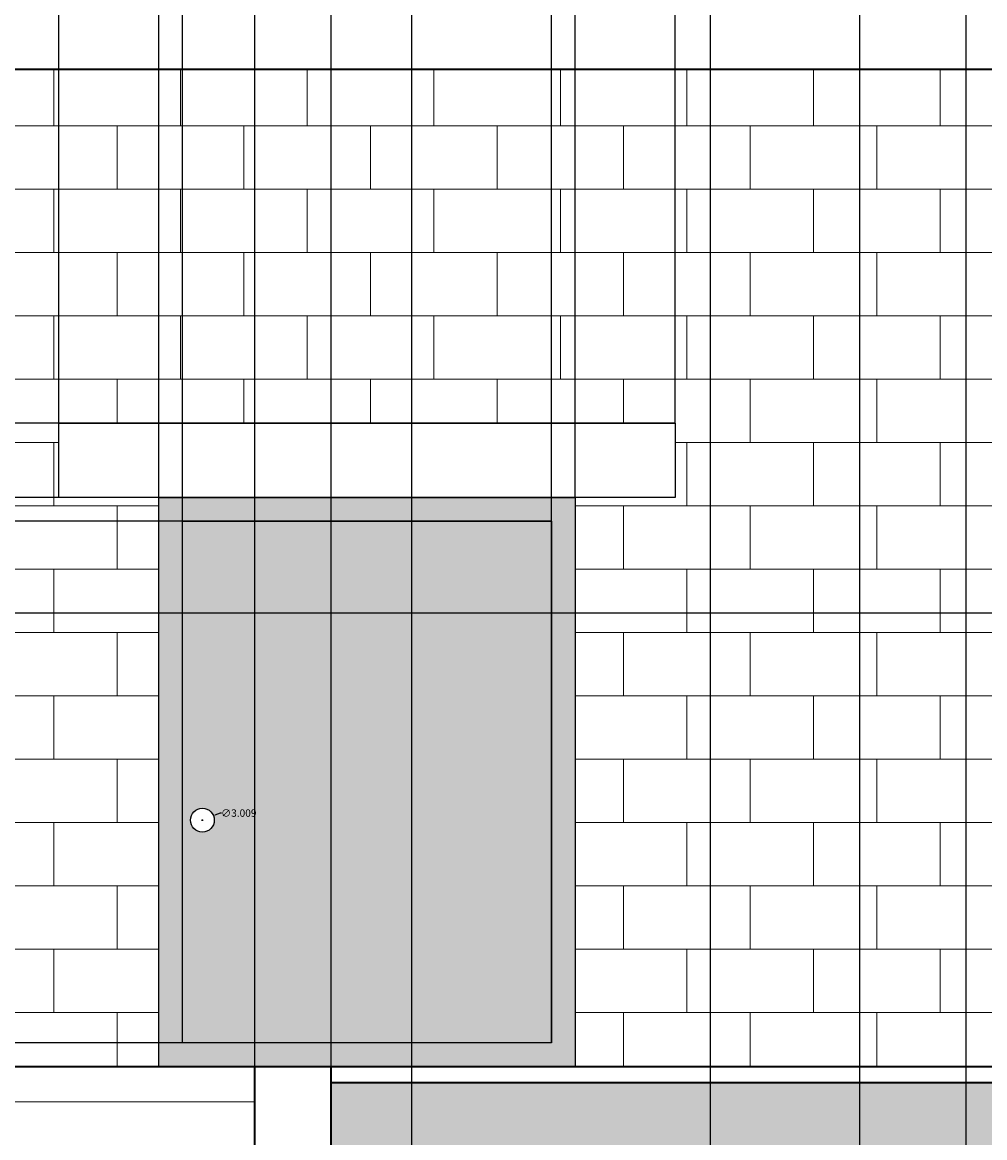
# Model space of a CAD drawing. Units: inches. Extents: x -5 to 714, y 84 to 644.
# Tile 11 of 20: x 220 to 342, y 336 to 477. Entities that reach past the tile are written whole.
import ezdxf

# ---------------------------------------------------------------- set-up
doc = ezdxf.new("R2010")
doc.units = ezdxf.units.IN
doc.header["$MEASUREMENT"] = 0
for name, color, linetype, lineweight in [('A-ANNO-DIMS', 2, 'Continuous', 18), ('A-DOOR', 4, 'Continuous', 25), ('A-ELEV', 7, 'Continuous', 35), ('A-ELEV-PATT', 8, 'Continuous', 13)]:
    doc.layers.add(name, color=color, linetype=linetype, lineweight=lineweight)
doc.styles.get("Standard").update_dxf_attribs({"font": 'arial.ttf'})
doc.dimstyles.get("Standard").update_dxf_attribs({"dimtxt": 0.9375, "dimasz": 0.18, "dimexe": 0.18, "dimexo": 0.0625, "dimgap": 0.09, "dimtad": 0, "dimtih": 1, "dimtoh": 1, "dimdec": 4, "dimzin": 0, "dimdsep": 46, "dimlunit": 4, "dimtxsty": 'Standard', "dimcen": 0.09, "dimadec": 0, "dimazin": 0, "dimtfac": 1, "dimtdec": 4, "dimtofl": 0, "dimtmove": 0, "dimatfit": 3, "dimfxl": 1, "dimtolj": 1, "dimtzin": 0, "dimarcsym": 0})

# ---------------------------------------------------------------- blocks, each defined once
blk = doc.blocks.new('*D27')
at = {"layer": 'A-ANNO-DIMS', "color": 0, "lineweight": -2, "transparency": 16777216}
for p, q in [((429.45, 402.48), (-2.74, 402.48)), ((-2.56, 402.3), (-2.56, 374.41)), ((-2.56, 345.37), (-2.56, 373.27)), ((429.45, 345.19), (-2.74, 345.19))]:
    blk.add_line(p, q, dxfattribs=at)
at = {"layer": 'A-ANNO-DIMS', "color": 0, "transparency": 16777216}
for points in [[(-2.59, 402.3), (-2.53, 402.3), (-2.56, 402.48)], [(-2.59, 345.37), (-2.53, 345.37), (-2.56, 345.19)]]:
    blk.add_solid(points, dxfattribs=at)
at = {"layer": 'Defpoints', "color": 0, "transparency": 16777216}
for p in [(-2.56, 402.48), (429.51, 402.48), (429.51, 345.19)]:
    blk.add_point(p, dxfattribs=at)
at = {"layer": 'A-ANNO-DIMS', "color": 0, "transparency": 16777216, "insert": (-2.56, 373.84), "char_height": 0.938, "attachment_point": 5}
blk.add_mtext('\\A1;57.29', dxfattribs=at)
blk = doc.blocks.new('*D29')
at = {"layer": 'A-ANNO-DIMS', "color": 0, "lineweight": -2, "transparency": 16777216}
for p, q in [((135.73, 471.11), (135.73, 84.31)), ((429.51, 471.11), (429.51, 84.31)), ((135.91, 84.49), (280.94, 84.49)), ((429.33, 84.49), (284.3, 84.49))]:
    blk.add_line(p, q, dxfattribs=at)
at = {"layer": 'A-ANNO-DIMS', "color": 0, "transparency": 16777216}
for points in [[(135.91, 84.52), (135.91, 84.46), (135.73, 84.49)], [(429.33, 84.52), (429.33, 84.46), (429.51, 84.49)]]:
    blk.add_solid(points, dxfattribs=at)
at = {"layer": 'Defpoints', "color": 0, "transparency": 16777216}
for p in [(135.73, 471.17), (429.51, 471.17), (429.51, 84.49)]:
    blk.add_point(p, dxfattribs=at)
at = {"layer": 'A-ANNO-DIMS', "color": 0, "transparency": 16777216, "insert": (282.62, 84.49), "char_height": 0.938, "attachment_point": 5}
blk.add_mtext('\\A1;293.8', dxfattribs=at)
blk = doc.blocks.new('*D31')
at = {"layer": 'A-ANNO-DIMS', "color": 0, "lineweight": -2, "transparency": 16777216}
for p, q in [((135.73, 345.26), (135.73, 643.61)), ((135.91, 643.43), (184.51, 643.43)), ((237.09, 643.43), (188.49, 643.43)), ((237.27, 345.26), (237.27, 643.61))]:
    blk.add_line(p, q, dxfattribs=at)
at = {"layer": 'A-ANNO-DIMS', "color": 0, "transparency": 16777216}
for points in [[(135.91, 643.46), (135.91, 643.4), (135.73, 643.43)], [(237.09, 643.46), (237.09, 643.4), (237.27, 643.43)]]:
    blk.add_solid(points, dxfattribs=at)
at = {"layer": 'Defpoints', "color": 0, "transparency": 16777216}
for p in [(237.27, 643.43), (135.73, 345.19), (237.27, 345.19)]:
    blk.add_point(p, dxfattribs=at)
at = {"layer": 'A-ANNO-DIMS', "color": 0, "transparency": 16777216, "insert": (186.5, 643.43), "char_height": 0.938, "attachment_point": 5}
blk.add_mtext('\\A1;101.54', dxfattribs=at)
blk = doc.blocks.new('*D32')
at = {"layer": 'A-ANNO-DIMS', "color": 0, "lineweight": -2, "transparency": 16777216}
for p, q in [((237.27, 417.15), (237.27, 643.61)), ((237.45, 643.43), (261.91, 643.43)), ((289.7, 643.43), (265.24, 643.43)), ((289.88, 417.15), (289.88, 643.61))]:
    blk.add_line(p, q, dxfattribs=at)
at = {"layer": 'A-ANNO-DIMS', "color": 0, "transparency": 16777216}
for points in [[(237.45, 643.46), (237.45, 643.4), (237.27, 643.43)], [(289.7, 643.46), (289.7, 643.4), (289.88, 643.43)]]:
    blk.add_solid(points, dxfattribs=at)
at = {"layer": 'Defpoints', "color": 0, "transparency": 16777216}
for p in [(289.88, 643.43), (237.27, 417.09), (289.88, 417.09)]:
    blk.add_point(p, dxfattribs=at)
at = {"layer": 'A-ANNO-DIMS', "color": 0, "transparency": 16777216, "insert": (263.57, 643.43), "char_height": 0.938, "attachment_point": 5}
blk.add_mtext('\\A1;52.62', dxfattribs=at)
blk = doc.blocks.new('*D33')
at = {"layer": 'A-ANNO-DIMS', "color": 0, "lineweight": -2, "transparency": 16777216}
for p, q in [((240.27, 348.26), (240.27, 643.61)), ((240.45, 643.43), (261.89, 643.43)), ((286.7, 643.43), (265.26, 643.43)), ((286.88, 348.26), (286.88, 643.61))]:
    blk.add_line(p, q, dxfattribs=at)
at = {"layer": 'A-ANNO-DIMS', "color": 0, "transparency": 16777216}
for points in [[(240.45, 643.46), (240.45, 643.4), (240.27, 643.43)], [(286.7, 643.46), (286.7, 643.4), (286.88, 643.43)]]:
    blk.add_solid(points, dxfattribs=at)
at = {"layer": 'Defpoints', "color": 0, "transparency": 16777216}
for p in [(286.88, 643.43), (240.27, 348.19), (286.88, 348.19)]:
    blk.add_point(p, dxfattribs=at)
at = {"layer": 'A-ANNO-DIMS', "color": 0, "transparency": 16777216, "insert": (263.57, 643.43), "char_height": 0.938, "attachment_point": 5}
blk.add_mtext('\\A1;46.62', dxfattribs=at)
blk = doc.blocks.new('*D34')
at = {"layer": 'A-ANNO-DIMS', "color": 0, "lineweight": -2, "transparency": 16777216}
for p, q in [((286.82, 414.09), (-2.74, 414.09)), ((-2.56, 413.91), (-2.56, 381.71)), ((-2.56, 348.37), (-2.56, 380.57)), ((286.82, 348.19), (-2.74, 348.19))]:
    blk.add_line(p, q, dxfattribs=at)
at = {"layer": 'A-ANNO-DIMS', "color": 0, "transparency": 16777216}
for points in [[(-2.59, 413.91), (-2.53, 413.91), (-2.56, 414.09)], [(-2.59, 348.37), (-2.53, 348.37), (-2.56, 348.19)]]:
    blk.add_solid(points, dxfattribs=at)
at = {"layer": 'Defpoints', "color": 0, "transparency": 16777216}
for p in [(-2.56, 414.09), (286.88, 414.09), (286.88, 348.19)]:
    blk.add_point(p, dxfattribs=at)
at = {"layer": 'A-ANNO-DIMS', "color": 0, "transparency": 16777216, "insert": (-2.56, 381.14), "char_height": 0.938, "attachment_point": 5}
blk.add_mtext('\\A1;65.9', dxfattribs=at)
blk = doc.blocks.new('*D35')
at = {"layer": 'A-ANNO-DIMS', "color": 0, "lineweight": -2, "transparency": 16777216}
for p, q in [((289.82, 417.09), (-2.74, 417.09)), ((-2.56, 416.91), (-2.56, 381.71)), ((-2.56, 345.37), (-2.56, 380.57)), ((289.82, 345.19), (-2.74, 345.19))]:
    blk.add_line(p, q, dxfattribs=at)
at = {"layer": 'A-ANNO-DIMS', "color": 0, "transparency": 16777216}
for points in [[(-2.59, 416.91), (-2.53, 416.91), (-2.56, 417.09)], [(-2.59, 345.37), (-2.53, 345.37), (-2.56, 345.19)]]:
    blk.add_solid(points, dxfattribs=at)
at = {"layer": 'Defpoints', "color": 0, "transparency": 16777216}
for p in [(-2.56, 417.09), (289.88, 417.09), (289.88, 345.19)]:
    blk.add_point(p, dxfattribs=at)
at = {"layer": 'A-ANNO-DIMS', "color": 0, "transparency": 16777216, "insert": (-2.56, 381.14), "char_height": 0.938, "attachment_point": 5}
blk.add_mtext('\\A1;71.9', dxfattribs=at)
blk = doc.blocks.new('*D36')
at = {"layer": 'A-ANNO-DIMS', "color": 0, "lineweight": -2, "transparency": 16777216}
for p, q in [((224.64, 426.51), (224.64, 643.61)), ((224.82, 643.43), (261.91, 643.43)), ((302.32, 643.43), (265.24, 643.43)), ((302.5, 426.51), (302.5, 643.61))]:
    blk.add_line(p, q, dxfattribs=at)
at = {"layer": 'A-ANNO-DIMS', "color": 0, "transparency": 16777216}
for points in [[(224.82, 643.46), (224.82, 643.4), (224.64, 643.43)], [(302.32, 643.46), (302.32, 643.4), (302.5, 643.43)]]:
    blk.add_solid(points, dxfattribs=at)
at = {"layer": 'Defpoints', "color": 0, "transparency": 16777216}
for p in [(302.5, 643.43), (224.64, 426.45), (302.5, 426.45)]:
    blk.add_point(p, dxfattribs=at)
at = {"layer": 'A-ANNO-DIMS', "color": 0, "transparency": 16777216, "insert": (263.57, 643.43), "char_height": 0.938, "attachment_point": 5}
blk.add_mtext('\\A1;77.86', dxfattribs=at)
blk = doc.blocks.new('*D37')
at = {"layer": 'A-ANNO-DIMS', "color": 0, "lineweight": -2, "transparency": 16777216}
for p, q in [((302.44, 426.45), (-2.74, 426.45)), ((-2.56, 426.27), (-2.56, 422.34)), ((-2.56, 417.27), (-2.56, 421.2)), ((302.44, 417.09), (-2.74, 417.09))]:
    blk.add_line(p, q, dxfattribs=at)
at = {"layer": 'A-ANNO-DIMS', "color": 0, "transparency": 16777216}
for points in [[(-2.59, 426.27), (-2.53, 426.27), (-2.56, 426.45)], [(-2.59, 417.27), (-2.53, 417.27), (-2.56, 417.09)]]:
    blk.add_solid(points, dxfattribs=at)
at = {"layer": 'Defpoints', "color": 0, "transparency": 16777216}
for p in [(-2.56, 426.45), (302.5, 426.45), (302.5, 417.09)]:
    blk.add_point(p, dxfattribs=at)
at = {"layer": 'A-ANNO-DIMS', "color": 0, "transparency": 16777216, "insert": (-2.56, 421.77), "char_height": 0.938, "attachment_point": 5}
blk.add_mtext('\\A1;9.358', dxfattribs=at)
blk = doc.blocks.new('*D51')
at = {"layer": 'A-ANNO-DIMS', "color": 0, "lineweight": -2, "transparency": 16777216}
for p, q in [((200.74, 201.26), (200.74, 643.61)), ((200.92, 643.43), (223.39, 643.43)), ((249.24, 643.43), (226.77, 643.43)), ((249.42, 201.26), (249.42, 643.61))]:
    blk.add_line(p, q, dxfattribs=at)
at = {"layer": 'A-ANNO-DIMS', "color": 0, "transparency": 16777216}
for points in [[(200.92, 643.46), (200.92, 643.4), (200.74, 643.43)], [(249.24, 643.46), (249.24, 643.4), (249.42, 643.43)]]:
    blk.add_solid(points, dxfattribs=at)
at = {"layer": 'Defpoints', "color": 0, "transparency": 16777216}
for p in [(249.42, 643.43), (200.74, 201.19), (249.42, 201.19)]:
    blk.add_point(p, dxfattribs=at)
at = {"layer": 'A-ANNO-DIMS', "color": 0, "transparency": 16777216, "insert": (225.08, 643.43), "char_height": 0.938, "attachment_point": 5}
blk.add_mtext('\\A1;48.68', dxfattribs=at)
blk = doc.blocks.new('*D52')
at = {"layer": 'A-ANNO-DIMS', "color": 0, "lineweight": -2, "transparency": 16777216}
for p, q in [((249.42, 345.13), (249.42, 84.31)), ((259.07, 345.13), (259.07, 84.31)), ((249.6, 84.49), (252.57, 84.49)), ((258.89, 84.49), (255.92, 84.49))]:
    blk.add_line(p, q, dxfattribs=at)
at = {"layer": 'A-ANNO-DIMS', "color": 0, "transparency": 16777216}
for points in [[(249.6, 84.52), (249.6, 84.46), (249.42, 84.49)], [(258.89, 84.52), (258.89, 84.46), (259.07, 84.49)]]:
    blk.add_solid(points, dxfattribs=at)
at = {"layer": 'Defpoints', "color": 0, "transparency": 16777216}
for p in [(249.42, 345.19), (259.07, 345.19), (259.07, 84.49)]:
    blk.add_point(p, dxfattribs=at)
at = {"layer": 'A-ANNO-DIMS', "color": 0, "transparency": 16777216, "insert": (254.24, 84.49), "char_height": 0.938, "attachment_point": 5}
blk.add_mtext('\\A1;9.648', dxfattribs=at)
blk = doc.blocks.new('*D54')
at = {"layer": 'A-ANNO-DIMS', "color": 0, "lineweight": -2, "transparency": 16777216}
for p, q in [((259.07, 315.16), (259.07, 643.61)), ((259.25, 643.43), (424.21, 643.43)), ((593.25, 643.43), (428.28, 643.43)), ((593.43, 315.16), (593.43, 643.61))]:
    blk.add_line(p, q, dxfattribs=at)
at = {"layer": 'A-ANNO-DIMS', "color": 0, "transparency": 16777216}
for points in [[(259.25, 643.46), (259.25, 643.4), (259.07, 643.43)], [(593.25, 643.46), (593.25, 643.4), (593.43, 643.43)]]:
    blk.add_solid(points, dxfattribs=at)
at = {"layer": 'Defpoints', "color": 0, "transparency": 16777216}
for p in [(593.43, 643.43), (259.07, 315.1), (593.43, 315.1)]:
    blk.add_point(p, dxfattribs=at)
at = {"layer": 'A-ANNO-DIMS', "color": 0, "transparency": 16777216, "insert": (426.25, 643.43), "char_height": 0.938, "attachment_point": 5}
blk.add_mtext('\\A1;334.36', dxfattribs=at)
blk = doc.blocks.new('*D60')
at = {"layer": 'A-ANNO-DIMS', "color": 0, "lineweight": -2, "transparency": 16777216}
for p, q in [((269.24, 277.11), (269.24, 643.61)), ((269.42, 643.43), (295.86, 643.43)), ((325.65, 643.43), (299.21, 643.43)), ((325.83, 266.06), (325.83, 643.61))]:
    blk.add_line(p, q, dxfattribs=at)
at = {"layer": 'A-ANNO-DIMS', "color": 0, "transparency": 16777216}
for points in [[(269.42, 643.46), (269.42, 643.4), (269.24, 643.43)], [(325.65, 643.46), (325.65, 643.4), (325.83, 643.43)]]:
    blk.add_solid(points, dxfattribs=at)
at = {"layer": 'Defpoints', "color": 0, "transparency": 16777216}
for p in [(325.83, 643.43), (269.24, 277.05), (325.83, 266)]:
    blk.add_point(p, dxfattribs=at)
at = {"layer": 'A-ANNO-DIMS', "color": 0, "transparency": 16777216, "insert": (297.54, 643.43), "char_height": 0.938, "attachment_point": 5}
blk.add_mtext('\\A1;56.59', dxfattribs=at)
blk = doc.blocks.new('*D61')
at = {"layer": 'A-ANNO-DIMS', "color": 0, "lineweight": -2, "transparency": 16777216}
for p, q in [((325.83, 266.06), (325.83, 643.61)), ((326.01, 643.43), (364.93, 643.43)), ((407.2, 643.43), (368.28, 643.43)), ((407.38, 266.06), (407.38, 643.61))]:
    blk.add_line(p, q, dxfattribs=at)
at = {"layer": 'A-ANNO-DIMS', "color": 0, "transparency": 16777216}
for points in [[(326.01, 643.46), (326.01, 643.4), (325.83, 643.43)], [(407.2, 643.46), (407.2, 643.4), (407.38, 643.43)]]:
    blk.add_solid(points, dxfattribs=at)
at = {"layer": 'Defpoints', "color": 0, "transparency": 16777216}
for p in [(407.38, 643.43), (325.83, 266), (407.38, 266)]:
    blk.add_point(p, dxfattribs=at)
at = {"layer": 'A-ANNO-DIMS', "color": 0, "transparency": 16777216, "insert": (366.61, 643.43), "char_height": 0.938, "attachment_point": 5}
blk.add_mtext('\\A1;81.55', dxfattribs=at)
blk = doc.blocks.new('*D83')
at = {"layer": 'A-ANNO-DIMS', "color": 0, "lineweight": -2, "transparency": 16777216}
for p, q in [((306.96, 144.93), (306.96, 643.61)), ((307.14, 643.43), (321.53, 643.43)), ((339.09, 643.43), (324.69, 643.43)), ((339.27, 144.93), (339.27, 643.61))]:
    blk.add_line(p, q, dxfattribs=at)
at = {"layer": 'A-ANNO-DIMS', "color": 0, "transparency": 16777216}
for points in [[(307.14, 643.46), (307.14, 643.4), (306.96, 643.43)], [(339.09, 643.46), (339.09, 643.4), (339.27, 643.43)]]:
    blk.add_solid(points, dxfattribs=at)
at = {"layer": 'Defpoints', "color": 0, "transparency": 16777216}
for p in [(339.27, 643.43), (306.96, 144.86), (339.27, 144.86)]:
    blk.add_point(p, dxfattribs=at)
at = {"layer": 'A-ANNO-DIMS', "color": 0, "transparency": 16777216, "insert": (323.11, 643.43), "char_height": 0.938, "attachment_point": 5}
blk.add_mtext('\\A1;32.31', dxfattribs=at)
blk = doc.blocks.new('*D94')
at = {"layer": 'A-ANNO-DIMS', "color": 0, "lineweight": -2, "transparency": 16777216}
for p, q in [((242.69, 376.31), (242.87, 376.31)), ((242.78, 376.22), (242.78, 376.4)), ((245.01, 377.21), (244.34, 376.94)), ((245.19, 377.21), (245.01, 377.21))]:
    blk.add_line(p, q, dxfattribs=at)
at = {"layer": 'A-ANNO-DIMS', "color": 0, "transparency": 16777216}
blk.add_solid([(244.33, 376.97), (244.36, 376.91), (244.18, 376.87)], dxfattribs=at)
at = {"layer": 'Defpoints', "color": 0, "transparency": 16777216}
for p in [(244.18, 376.87), (241.39, 375.75)]:
    blk.add_point(p, dxfattribs=at)
at = {"layer": 'A-ANNO-DIMS', "color": 0, "transparency": 16777216, "insert": (247.38, 377.21), "char_height": 0.938, "attachment_point": 5}
blk.add_mtext('\\A1;∅3.009', dxfattribs=at)

msp = doc.modelspace()

# ---------------------------------------------------------------- hatches: boundary and pattern name
at = {"layer": 'A-ELEV-PATT', "transparency": 33554687}
h = msp.add_hatch(dxfattribs=at)
h.set_pattern_fill('ANSI31', color=256, scale=58, angle=135)
h.paths.add_polyline_path([(249.4181, 345.1928), (237.2654, 345.1928), (200.7361, 345.1928), (200.7361, 201.1928), (249.4181, 201.1928)])
h.paths.add_polyline_path([(261.4349, 199.1928), (189.6349, 199.1928), (189.6349, 154.1176), (261.4349, 154.1176)])
h.paths.add_polyline_path([(415.8092, 525.1928), (366.2809, 525.1928), (366.2809, 480.1709), (415.8092, 480.1709)])
h = msp.add_hatch(dxfattribs=at)
h.set_pattern_fill('AR-B816', color=256)
h.paths.add_polyline_path([(429.5094, 471.1709), (412.7784, 471.1709), (229.3575, 471.1709), (135.7303, 471.1709), (135.7303, 345.1928), (237.2654, 345.1928), (237.2654, 417.0908), (224.6446, 417.0908), (224.6446, 426.4485), (302.5023, 426.4485), (302.5023, 417.0908), (289.8815, 417.0908), (289.8815, 345.1928), (429.5094, 345.1928)])
h = msp.add_hatch(color=256, dxfattribs=at)
h.dxf.hatch_style = 1
h.paths.add_polyline_path([(289.8815, 417.0908), (237.2654, 417.0908), (237.2654, 345.1928), (289.8815, 345.1928)])
h.paths.add_polyline_path([(286.8815, 414.0908), (286.8815, 348.1928), (240.2654, 348.1928), (240.2654, 414.0908)], flags=16)
h.paths.add_polyline_path([(244.2856, 376.3091, -1), (241.2767, 376.3091, -1)], flags=0)
h.paths.add_polyline_path([(543.7164, 266.0021), (493.7771, 266.0021), (493.7771, 201.1928), (499.6809, 201.1928), (499.6809, 257.3379), (537.1779, 257.3379), (537.1779, 201.1928), (543.7164, 201.1928)])
h = msp.add_hatch(color=256, dxfattribs=at)
h.dxf.hatch_style = 1
h.paths.add_polyline_path([(286.8815, 414.0908), (240.2654, 414.0908), (240.2654, 348.1928), (286.8815, 348.1928)])
h.paths.add_polyline_path([(244.2856, 376.3091, -1), (241.2767, 376.3091, -1)], flags=16)
h = msp.add_hatch(color=256, dxfattribs=at)
h.dxf.hatch_style = 1
h.paths.add_polyline_path([(584.2229, 343.1928), (259.0665, 343.1928), (259.0665, 315.0968), (584.2229, 315.0968)])
h.paths.add_polyline_path([(352.9482, 258.2864), (332.0052, 258.2864), (332.0052, 201.1928), (352.9482, 201.1928)])
h.paths.add_polyline_path([(378.5957, 258.2864), (357.6527, 258.2864), (357.6527, 201.1928), (378.5957, 201.1928)])
h.paths.add_polyline_path([(403.4391, 258.2864), (382.4961, 258.2864), (382.4961, 201.1928), (403.4391, 201.1928)])
h.paths.add_polyline_path([(339.2672, 197.3754), (332.0052, 197.3754), (332.0052, 191.3028), (339.2672, 191.3028)])
h.paths.add_polyline_path([(352.9482, 197.3754), (343.9704, 197.3754), (343.9704, 191.3028), (352.9482, 191.3028)])
h.paths.add_polyline_path([(352.9482, 189.3028), (343.9704, 189.3028), (343.9704, 184.8307), (352.9482, 184.8307)])
h.paths.add_polyline_path([(339.2672, 189.3028), (332.0052, 189.3028), (332.0052, 184.8307), (339.2672, 184.8307)])
h.paths.add_polyline_path([(339.2672, 182.8307), (332.0052, 182.8307), (332.0052, 177.6504), (339.2672, 177.6504)])
h.paths.add_polyline_path([(352.9482, 182.8307), (343.9704, 182.8307), (343.9704, 177.6504), (352.9482, 177.6504)])
h.paths.add_polyline_path([(352.9482, 175.6504), (343.9704, 175.6504), (343.9704, 173.6169), (352.9482, 173.6169)])
h.paths.add_polyline_path([(339.2672, 175.6504), (332.0052, 175.6504), (332.0052, 173.6169), (339.2672, 173.6169)])
h.paths.add_polyline_path([(376.2796, 175.6504), (357.6527, 175.6504), (357.6527, 173.6169), (376.2796, 173.6169)])
h.paths.add_polyline_path([(376.2796, 182.8307), (357.6527, 182.8307), (357.6527, 177.6504), (376.2796, 177.6504)])
h.paths.add_polyline_path([(376.2796, 189.3028), (357.6527, 189.3028), (357.6527, 184.8307), (376.2796, 184.8307)])
h.paths.add_polyline_path([(376.2796, 197.3754), (357.6527, 197.3754), (357.6527, 191.3028), (376.2796, 191.3028)])
h.paths.add_polyline_path([(403.4391, 197.3754), (382.4961, 197.3754), (382.4961, 191.3028), (403.4391, 191.3028)])
h.paths.add_polyline_path([(403.4391, 189.3028), (382.4961, 189.3028), (382.4961, 184.8307), (403.4391, 184.8307)])
h.paths.add_polyline_path([(403.4391, 182.8307), (382.4961, 182.8307), (382.4961, 177.6504), (403.4391, 177.6504)])
h.paths.add_polyline_path([(403.4391, 175.6504), (382.4961, 175.6504), (382.4961, 173.6169), (403.4391, 173.6169)])

# ---------------------------------------------------------------- linework, layer by layer
at = {"layer": 'A-DOOR'}
for points in [[(224.6446, 426.4485), (302.5023, 426.4485), (302.5023, 417.0908), (224.6446, 417.0908)], [(237.2654, 417.0908), (289.8815, 417.0908), (289.8815, 345.1928), (237.2654, 345.1928)], [(240.2654, 414.0908), (286.8815, 414.0908), (286.8815, 348.1928), (240.2654, 348.1928)]]:
    msp.add_lwpolyline(points, close=True, dxfattribs=at)
msp.add_circle((242.7811, 376.3091), 1.5044, dxfattribs=at)
at = {"layer": 'A-ELEV'}
for p, q in [((135.7303, 471.1709), (229.3575, 471.1709)), ((229.3575, 471.1709), (412.7784, 471.1709)), ((67.9893, 345.1928), (587.5794, 345.1928)), ((249.4181, 201.1928), (249.4181, 345.1928)), ((259.0665, 201.1928), (259.0665, 345.1928)), ((259.0665, 343.1928), (584.2229, 343.1928))]:
    msp.add_line(p, q, dxfattribs=at)

# ---------------------------------------------------------------- dimensions: what is measured, and where the dimension line sits
at = {"layer": 'A-ANNO-DIMS'}
for base, p1, p2, override, picture, middle in [((237.2654, 643.4276), (135.7303, 345.1928), (237.2654, 345.1928), {"dimdec": 2, "dimlfac": 1, "dimrnd": 0, "dimzin": 0, "dimdsep": 46, "dimlunit": 2}, '*D31', (186.4978, 643.4276)), ((249.4181, 643.4276), (200.7361, 201.1928), (249.4181, 201.1928), {"dimdec": 2, "dimlfac": 1, "dimrnd": 0, "dimzin": 0, "dimdsep": 46, "dimlunit": 2}, '*D51', (225.0771, 643.4276)), ((302.5023, 643.4276), (224.6446, 426.4485), (302.5023, 426.4485), {"dimdec": 2, "dimlfac": 1, "dimrnd": 0, "dimzin": 0, "dimdsep": 46, "dimlunit": 2}, '*D36', (263.5734, 643.4276)), ((289.8815, 643.4276), (237.2654, 417.0908), (289.8815, 417.0908), {"dimdec": 2, "dimlfac": 1, "dimrnd": 0, "dimzin": 0, "dimdsep": 46, "dimlunit": 2}, '*D32', (263.5734, 643.4276)), ((286.8815, 643.4276), (240.2654, 348.1928), (286.8815, 348.1928), {"dimdec": 2, "dimlfac": 1, "dimrnd": 0, "dimzin": 0, "dimdsep": 46, "dimlunit": 2}, '*D33', (263.5734, 643.4276)), ((593.428, 643.4276), (259.0665, 315.0968), (593.428, 315.0968), {"dimdec": 2, "dimlfac": 1, "dimrnd": 0, "dimzin": 0, "dimdsep": 46, "dimlunit": 2}, '*D54', (426.2472, 643.4276)), ((325.8305, 643.4276), (269.2446, 277.0513), (325.8305, 266.0021), {"dimdec": 2, "dimlfac": 1, "dimrnd": 0, "dimzin": 0, "dimdsep": 46, "dimlunit": 2}, '*D60', (297.5375, 643.4276)), ((339.2672, 643.4276), (306.958, 144.8639), (339.2672, 144.8639), {"dimdec": 2, "dimlfac": 1, "dimrnd": 0, "dimzin": 0, "dimdsep": 46, "dimlunit": 2}, '*D83', (323.1126, 643.4276)), ((407.3813, 643.4276), (325.8305, 266.0021), (407.3813, 266.0021), {"dimdec": 2, "dimlfac": 1, "dimrnd": 0, "dimzin": 0, "dimdsep": 46, "dimlunit": 2}, '*D61', (366.6059, 643.4276)), ((429.5094, 84.4928), (135.7303, 471.1709), (429.5094, 471.1709), {"dimdec": 1, "dimlfac": 1, "dimrnd": 0, "dimzin": 0, "dimdsep": 46, "dimlunit": 2}, '*D29', (282.6198, 84.4928)), ((259.0665, 84.4928), (249.4181, 345.1928), (259.0665, 345.1928), {"dimdec": 3, "dimlfac": 1, "dimrnd": 0, "dimzin": 0, "dimdsep": 46, "dimlunit": 2}, '*D52', (254.2423, 84.4928))]:
    dim = msp.add_linear_dim(base=base, p1=p1, p2=p2, dimstyle='Standard', override=override, dxfattribs=at)
    dim.commit()
    dim.dimension.update_dxf_attribs({"geometry": picture, "text_midpoint": middle})
for base, p1, p2, override, picture, middle in [((-2.5605, 426.4485), (302.5023, 417.0908), (302.5023, 426.4485), {"dimdec": 3, "dimlfac": 1, "dimrnd": 0, "dimzin": 0, "dimdsep": 46, "dimlunit": 2}, '*D37', (-2.5605, 421.7696)), ((-2.5605, 417.0908), (289.8815, 345.1928), (289.8815, 417.0908), {"dimdec": 1, "dimlfac": 1, "dimrnd": 0, "dimzin": 0, "dimdsep": 46, "dimlunit": 2}, '*D35', (-2.5605, 381.1418)), ((-2.5605, 414.0908), (286.8815, 348.1928), (286.8815, 414.0908), {"dimdec": 1, "dimlfac": 1, "dimrnd": 0, "dimzin": 0, "dimdsep": 46, "dimlunit": 2}, '*D34', (-2.5605, 381.1418)), ((-2.5605, 402.4806), (429.5094, 345.1928), (429.5094, 402.4806), {"dimdec": 2, "dimlfac": 1, "dimrnd": 0, "dimzin": 0, "dimdsep": 46, "dimlunit": 2}, '*D27', (-2.5605, 373.8367))]:
    dim = msp.add_linear_dim(base=base, p1=p1, p2=p2, angle=90, dimstyle='Standard', override=override, dxfattribs=at)
    dim.commit()
    dim.dimension.update_dxf_attribs({"geometry": picture, "text_midpoint": middle})
dim = msp.add_diameter_dim_2p(p1=(241.3853, 375.748), p2=(244.177, 376.8702), dimstyle='Standard', override={"dimdec": 3, "dimlfac": 1, "dimrnd": 0, "dimzin": 0, "dimdsep": 46, "dimlunit": 2}, dxfattribs=at)
dim.commit()
dim.dimension.update_dxf_attribs({"geometry": '*D94', "text_midpoint": (247.3773, 377.2068), "dimtype": 163})

doc.saveas('drawing.dxf')
